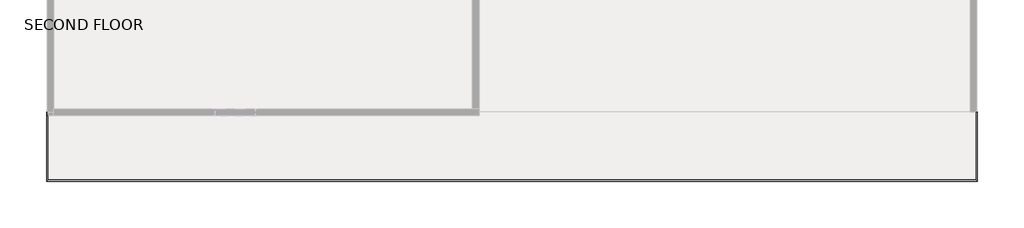
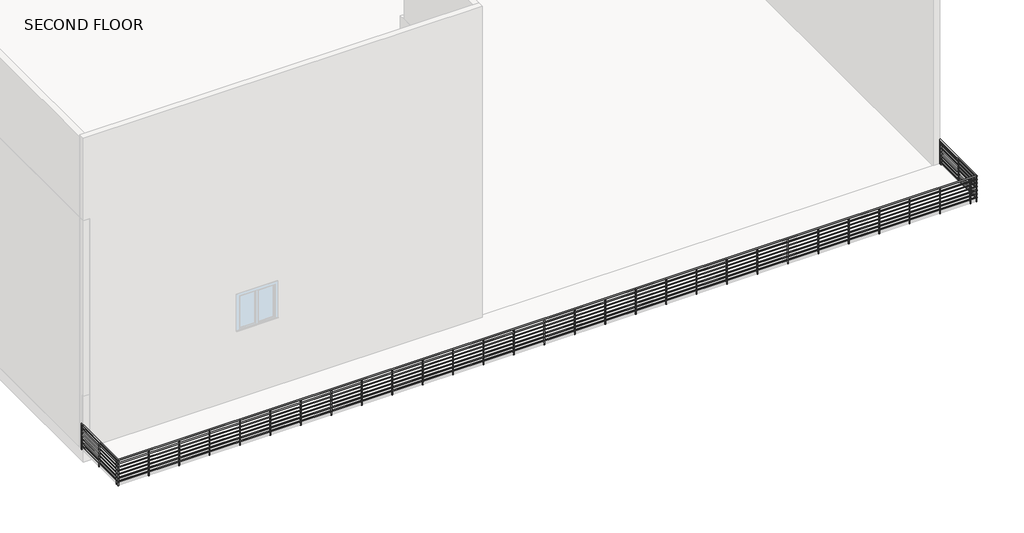
# One storey, part 2 of 2: 1 railing.
"""IFC4 building model written with IfcOpenShell, lengths in millimetres."""

from ifc_helpers import new_model, si_unit, point, frame, frame_2d, origin, place, context, project, spatial, circle_curve, ellipse_curve, trimmed, segment, composite_curve, outline, extrude, element, save
from ifc_brep_helpers import plane_surface, cylinder_surface, advanced_brep

model = new_model("IFC4")

# Units and contexts
model_context = context("Model", 3, world=origin())
ifc_project = project(units=[si_unit("LENGTHUNIT", "METRE", prefix="MILLI")], contexts=[model_context])

# Site, building, storey
site = spatial("IfcSite", under=ifc_project)
building = spatial("IfcBuilding", under=site)
storey = spatial("IfcBuildingStorey", under=building, Name="SECOND FLOOR", Elevation=6096.0)

# Railing
placement = place(None, origin())
element("IfcRailing", 1, ObjectType="900mm Pipe", at=placement, inside=storey, context=model_context, shape_type="SolidModel", body=[
    advanced_brep(
    [(-17910.01982, -7832.8965627, 6976.0), (-17870.01982, -7832.8965627, 6976.0), (-17910.01982, -9933.0763423, 6976.0), (-17870.01982, -9893.0763423, 6976.0), (10329.98018, -9933.0763423, 6976.0), (10289.98018, -9893.0763423, 6976.0), (10329.98018, -7832.8965627, 6976.0), (10289.98018, -7832.8965627, 6976.0)],
    [
        (0, 1, circle_curve(frame((-17890.01982, -7832.8965627, 6976.0), z_axis=(0.0, 1.0, 0.0), x_axis=(1.0, 0.0, 0.0)), 20.0)),
        (1, 0, circle_curve(frame((-17890.01982, -7832.8965627, 6976.0), z_axis=(0.0, 1.0, 0.0), x_axis=(1.0, 0.0, 0.0)), 20.0)),
        (0, 2),
        (2, 3, ellipse_curve(frame((-17890.01982, -9913.0763423, 6976.0), z_axis=(-0.7071067811865475, 0.7071067811865475, 0.0), x_axis=(0.7071067811865474, 0.7071067811865476, 0.0)), 28.2842712, 20.0)),
        (3, 1),
        (3, 2, ellipse_curve(frame((-17890.01982, -9913.0763423, 6976.0), z_axis=(-0.7071067811865475, 0.7071067811865475, 0.0), x_axis=(0.7071067811865474, 0.7071067811865476, 0.0)), 28.2842712, 20.0)),
        (2, 4),
        (4, 5, ellipse_curve(frame((10309.98018, -9913.0763423, 6976.0), z_axis=(-0.7071067811865475, -0.7071067811865475, 0.0), x_axis=(-0.7071067811865476, 0.7071067811865474, 0.0)), 28.2842712, 20.0)),
        (5, 3),
        (5, 4, ellipse_curve(frame((10309.98018, -9913.0763423, 6976.0), z_axis=(-0.7071067811865475, -0.7071067811865475, 0.0), x_axis=(-0.7071067811865476, 0.7071067811865474, 0.0)), 28.2842712, 20.0)),
        (6, 7, circle_curve(frame((10309.98018, -7832.8965627, 6976.0), z_axis=(0.0, 1.0, 0.0), x_axis=(-1.0, 0.0, 0.0)), 20.0)),
        (7, 6, circle_curve(frame((10309.98018, -7832.8965627, 6976.0), z_axis=(0.0, 1.0, 0.0), x_axis=(-1.0, 0.0, 0.0)), 20.0)),
        (4, 6),
        (7, 5),
    ],
    [
        plane_surface(frame((-17890.01982, -7832.8965627, 6996.0), z_axis=(0.0, 1.0, 0.0), x_axis=(0.0, 0.0, -1.0))),
        cylinder_surface(frame((-17890.01982, -7832.8965627, 6976.0), z_axis=(0.0, 1.0, 0.0), x_axis=(1.0, 0.0, 0.0)), 20.0),
        cylinder_surface(frame((-17890.01982, -9913.0763423, 6976.0), z_axis=(-1.0, 0.0, 0.0), x_axis=(0.0, 1.0, 0.0)), 20.0),
        plane_surface(frame((10309.98018, -7832.8965627, 6996.0), z_axis=(0.0, 1.0, 0.0), x_axis=(0.0, 0.0, 1.0))),
        cylinder_surface(frame((10309.98018, -9913.0763423, 6976.0), z_axis=(0.0, -1.0, 0.0), x_axis=(-1.0, 0.0, 0.0)), 20.0),
    ],
    [
        (0, [[1, 2]]),
        (1, [[-1, 3, 4, 5]]),
        (1, [[-2, -5, 6, -3]]),
        (2, [[-4, 7, 8, 9]]),
        (2, [[-6, -9, 10, -7]]),
        (3, [[11, 12]]),
        (4, [[-8, 13, -12, 14]]),
        (4, [[-10, -14, -11, -13]]),
    ],
),
    advanced_brep(
    [(-17875.01982, -7832.8965627, 6856.0), (-17905.01982, -7832.8965627, 6856.0), (-17875.01982, -9898.0763423, 6856.0), (-17905.01982, -9928.0763423, 6856.0), (10294.98018, -9898.0763423, 6856.0), (10324.98018, -9928.0763423, 6856.0), (10294.98018, -7832.8965627, 6856.0), (10324.98018, -7832.8965627, 6856.0)],
    [
        (0, 1, circle_curve(frame((-17890.01982, -7832.8965627, 6856.0), z_axis=(0.0, 1.0, 0.0), x_axis=(-1.0, 0.0, 0.0)), 15.0)),
        (1, 0, circle_curve(frame((-17890.01982, -7832.8965627, 6856.0), z_axis=(0.0, 1.0, 0.0), x_axis=(-1.0, 0.0, 0.0)), 15.0)),
        (0, 2),
        (2, 3, ellipse_curve(frame((-17890.01982, -9913.0763423, 6856.0), z_axis=(-0.7071067811865475, 0.7071067811865475, 0.0), x_axis=(0.7071067811865474, 0.7071067811865476, 0.0)), 21.2132034, 15.0)),
        (3, 1),
        (3, 2, ellipse_curve(frame((-17890.01982, -9913.0763423, 6856.0), z_axis=(-0.7071067811865475, 0.7071067811865475, 0.0), x_axis=(0.7071067811865474, 0.7071067811865476, 0.0)), 21.2132034, 15.0)),
        (2, 4),
        (4, 5, ellipse_curve(frame((10309.98018, -9913.0763423, 6856.0), z_axis=(-0.7071067811865475, -0.7071067811865475, 0.0), x_axis=(-0.7071067811865476, 0.7071067811865474, 0.0)), 21.2132034, 15.0)),
        (5, 3),
        (5, 4, ellipse_curve(frame((10309.98018, -9913.0763423, 6856.0), z_axis=(-0.7071067811865475, -0.7071067811865475, 0.0), x_axis=(-0.7071067811865476, 0.7071067811865474, 0.0)), 21.2132034, 15.0)),
        (6, 7, circle_curve(frame((10309.98018, -7832.8965627, 6856.0), z_axis=(0.0, 1.0, 0.0), x_axis=(1.0, 0.0, 0.0)), 15.0)),
        (7, 6, circle_curve(frame((10309.98018, -7832.8965627, 6856.0), z_axis=(0.0, 1.0, 0.0), x_axis=(1.0, 0.0, 0.0)), 15.0)),
        (4, 6),
        (7, 5),
    ],
    [
        plane_surface(frame((-17890.01982, -7832.8965627, 6871.0), z_axis=(0.0, 1.0, 0.0), x_axis=(0.0, 0.0, -1.0))),
        cylinder_surface(frame((-17890.01982, -7832.8965627, 6856.0), z_axis=(0.0, 1.0, 0.0), x_axis=(-1.0, 0.0, 0.0)), 15.0),
        cylinder_surface(frame((-17890.01982, -9913.0763423, 6856.0), z_axis=(-1.0, 0.0, 0.0), x_axis=(0.0, -1.0, 0.0)), 15.0),
        plane_surface(frame((10309.98018, -7832.8965627, 6871.0), z_axis=(0.0, 1.0, 0.0), x_axis=(0.0, 0.0, 1.0))),
        cylinder_surface(frame((10309.98018, -9913.0763423, 6856.0), z_axis=(0.0, -1.0, 0.0), x_axis=(1.0, 0.0, 0.0)), 15.0),
    ],
    [
        (0, [[1, 2]]),
        (1, [[-1, 3, 4, 5]]),
        (1, [[-2, -5, 6, -3]]),
        (2, [[-4, 7, 8, 9]]),
        (2, [[-6, -9, 10, -7]]),
        (3, [[11, 12]]),
        (4, [[-8, 13, -12, 14]]),
        (4, [[-10, -14, -11, -13]]),
    ],
),
    advanced_brep(
    [(-17875.01982, -7832.8965627, 6731.0), (-17905.01982, -7832.8965627, 6731.0), (-17875.01982, -9898.0763423, 6731.0), (-17905.01982, -9928.0763423, 6731.0), (10294.98018, -9898.0763423, 6731.0), (10324.98018, -9928.0763423, 6731.0), (10294.98018, -7832.8965627, 6731.0), (10324.98018, -7832.8965627, 6731.0)],
    [
        (0, 1, circle_curve(frame((-17890.01982, -7832.8965627, 6731.0), z_axis=(0.0, 1.0, 0.0), x_axis=(-1.0, 0.0, 0.0)), 15.0)),
        (1, 0, circle_curve(frame((-17890.01982, -7832.8965627, 6731.0), z_axis=(0.0, 1.0, 0.0), x_axis=(-1.0, 0.0, 0.0)), 15.0)),
        (0, 2),
        (2, 3, ellipse_curve(frame((-17890.01982, -9913.0763423, 6731.0), z_axis=(-0.7071067811865475, 0.7071067811865475, 0.0), x_axis=(0.7071067811865474, 0.7071067811865476, 0.0)), 21.2132034, 15.0)),
        (3, 1),
        (3, 2, ellipse_curve(frame((-17890.01982, -9913.0763423, 6731.0), z_axis=(-0.7071067811865475, 0.7071067811865475, 0.0), x_axis=(0.7071067811865474, 0.7071067811865476, 0.0)), 21.2132034, 15.0)),
        (2, 4),
        (4, 5, ellipse_curve(frame((10309.98018, -9913.0763423, 6731.0), z_axis=(-0.7071067811865475, -0.7071067811865475, 0.0), x_axis=(-0.7071067811865476, 0.7071067811865474, 0.0)), 21.2132034, 15.0)),
        (5, 3),
        (5, 4, ellipse_curve(frame((10309.98018, -9913.0763423, 6731.0), z_axis=(-0.7071067811865475, -0.7071067811865475, 0.0), x_axis=(-0.7071067811865476, 0.7071067811865474, 0.0)), 21.2132034, 15.0)),
        (6, 7, circle_curve(frame((10309.98018, -7832.8965627, 6731.0), z_axis=(0.0, 1.0, 0.0), x_axis=(1.0, 0.0, 0.0)), 15.0)),
        (7, 6, circle_curve(frame((10309.98018, -7832.8965627, 6731.0), z_axis=(0.0, 1.0, 0.0), x_axis=(1.0, 0.0, 0.0)), 15.0)),
        (4, 6),
        (7, 5),
    ],
    [
        plane_surface(frame((-17890.01982, -7832.8965627, 6746.0), z_axis=(0.0, 1.0, 0.0), x_axis=(0.0, 0.0, -1.0))),
        cylinder_surface(frame((-17890.01982, -7832.8965627, 6731.0), z_axis=(0.0, 1.0, 0.0), x_axis=(-1.0, 0.0, 0.0)), 15.0),
        cylinder_surface(frame((-17890.01982, -9913.0763423, 6731.0), z_axis=(-1.0, 0.0, 0.0), x_axis=(0.0, -1.0, 0.0)), 15.0),
        plane_surface(frame((10309.98018, -7832.8965627, 6746.0), z_axis=(0.0, 1.0, 0.0), x_axis=(0.0, 0.0, 1.0))),
        cylinder_surface(frame((10309.98018, -9913.0763423, 6731.0), z_axis=(0.0, -1.0, 0.0), x_axis=(1.0, 0.0, 0.0)), 15.0),
    ],
    [
        (0, [[1, 2]]),
        (1, [[-1, 3, 4, 5]]),
        (1, [[-2, -5, 6, -3]]),
        (2, [[-4, 7, 8, 9]]),
        (2, [[-6, -9, 10, -7]]),
        (3, [[11, 12]]),
        (4, [[-8, 13, -12, 14]]),
        (4, [[-10, -14, -11, -13]]),
    ],
),
    advanced_brep(
    [(-17875.01982, -7832.8965627, 6606.0), (-17905.01982, -7832.8965627, 6606.0), (-17875.01982, -9898.0763423, 6606.0), (-17905.01982, -9928.0763423, 6606.0), (10294.98018, -9898.0763423, 6606.0), (10324.98018, -9928.0763423, 6606.0), (10294.98018, -7832.8965627, 6606.0), (10324.98018, -7832.8965627, 6606.0)],
    [
        (0, 1, circle_curve(frame((-17890.01982, -7832.8965627, 6606.0), z_axis=(0.0, 1.0, 0.0), x_axis=(-1.0, 0.0, 0.0)), 15.0)),
        (1, 0, circle_curve(frame((-17890.01982, -7832.8965627, 6606.0), z_axis=(0.0, 1.0, 0.0), x_axis=(-1.0, 0.0, 0.0)), 15.0)),
        (0, 2),
        (2, 3, ellipse_curve(frame((-17890.01982, -9913.0763423, 6606.0), z_axis=(-0.7071067811865475, 0.7071067811865475, 0.0), x_axis=(0.7071067811865474, 0.7071067811865476, 0.0)), 21.2132034, 15.0)),
        (3, 1),
        (3, 2, ellipse_curve(frame((-17890.01982, -9913.0763423, 6606.0), z_axis=(-0.7071067811865475, 0.7071067811865475, 0.0), x_axis=(0.7071067811865474, 0.7071067811865476, 0.0)), 21.2132034, 15.0)),
        (2, 4),
        (4, 5, ellipse_curve(frame((10309.98018, -9913.0763423, 6606.0), z_axis=(-0.7071067811865475, -0.7071067811865475, 0.0), x_axis=(-0.7071067811865476, 0.7071067811865474, 0.0)), 21.2132034, 15.0)),
        (5, 3),
        (5, 4, ellipse_curve(frame((10309.98018, -9913.0763423, 6606.0), z_axis=(-0.7071067811865475, -0.7071067811865475, 0.0), x_axis=(-0.7071067811865476, 0.7071067811865474, 0.0)), 21.2132034, 15.0)),
        (6, 7, circle_curve(frame((10309.98018, -7832.8965627, 6606.0), z_axis=(0.0, 1.0, 0.0), x_axis=(1.0, 0.0, 0.0)), 15.0)),
        (7, 6, circle_curve(frame((10309.98018, -7832.8965627, 6606.0), z_axis=(0.0, 1.0, 0.0), x_axis=(1.0, 0.0, 0.0)), 15.0)),
        (4, 6),
        (7, 5),
    ],
    [
        plane_surface(frame((-17890.01982, -7832.8965627, 6621.0), z_axis=(0.0, 1.0, 0.0), x_axis=(0.0, 0.0, -1.0))),
        cylinder_surface(frame((-17890.01982, -7832.8965627, 6606.0), z_axis=(0.0, 1.0, 0.0), x_axis=(-1.0, 0.0, 0.0)), 15.0),
        cylinder_surface(frame((-17890.01982, -9913.0763423, 6606.0), z_axis=(-1.0, 0.0, 0.0), x_axis=(0.0, -1.0, 0.0)), 15.0),
        plane_surface(frame((10309.98018, -7832.8965627, 6621.0), z_axis=(0.0, 1.0, 0.0), x_axis=(0.0, 0.0, 1.0))),
        cylinder_surface(frame((10309.98018, -9913.0763423, 6606.0), z_axis=(0.0, -1.0, 0.0), x_axis=(1.0, 0.0, 0.0)), 15.0),
    ],
    [
        (0, [[1, 2]]),
        (1, [[-1, 3, 4, 5]]),
        (1, [[-2, -5, 6, -3]]),
        (2, [[-4, 7, 8, 9]]),
        (2, [[-6, -9, 10, -7]]),
        (3, [[11, 12]]),
        (4, [[-8, 13, -12, 14]]),
        (4, [[-10, -14, -11, -13]]),
    ],
),
    advanced_brep(
    [(-17875.01982, -7832.8965627, 6481.0), (-17905.01982, -7832.8965627, 6481.0), (-17875.01982, -9898.0763423, 6481.0), (-17905.01982, -9928.0763423, 6481.0), (10294.98018, -9898.0763423, 6481.0), (10324.98018, -9928.0763423, 6481.0), (10294.98018, -7832.8965627, 6481.0), (10324.98018, -7832.8965627, 6481.0)],
    [
        (0, 1, circle_curve(frame((-17890.01982, -7832.8965627, 6481.0), z_axis=(0.0, 1.0, 0.0), x_axis=(-1.0, 0.0, 0.0)), 15.0)),
        (1, 0, circle_curve(frame((-17890.01982, -7832.8965627, 6481.0), z_axis=(0.0, 1.0, 0.0), x_axis=(-1.0, 0.0, 0.0)), 15.0)),
        (0, 2),
        (2, 3, ellipse_curve(frame((-17890.01982, -9913.0763423, 6481.0), z_axis=(-0.7071067811865475, 0.7071067811865475, 0.0), x_axis=(0.7071067811865474, 0.7071067811865476, 0.0)), 21.2132034, 15.0)),
        (3, 1),
        (3, 2, ellipse_curve(frame((-17890.01982, -9913.0763423, 6481.0), z_axis=(-0.7071067811865475, 0.7071067811865475, 0.0), x_axis=(0.7071067811865474, 0.7071067811865476, 0.0)), 21.2132034, 15.0)),
        (2, 4),
        (4, 5, ellipse_curve(frame((10309.98018, -9913.0763423, 6481.0), z_axis=(-0.7071067811865475, -0.7071067811865475, 0.0), x_axis=(-0.7071067811865476, 0.7071067811865474, 0.0)), 21.2132034, 15.0)),
        (5, 3),
        (5, 4, ellipse_curve(frame((10309.98018, -9913.0763423, 6481.0), z_axis=(-0.7071067811865475, -0.7071067811865475, 0.0), x_axis=(-0.7071067811865476, 0.7071067811865474, 0.0)), 21.2132034, 15.0)),
        (6, 7, circle_curve(frame((10309.98018, -7832.8965627, 6481.0), z_axis=(0.0, 1.0, 0.0), x_axis=(1.0, 0.0, 0.0)), 15.0)),
        (7, 6, circle_curve(frame((10309.98018, -7832.8965627, 6481.0), z_axis=(0.0, 1.0, 0.0), x_axis=(1.0, 0.0, 0.0)), 15.0)),
        (4, 6),
        (7, 5),
    ],
    [
        plane_surface(frame((-17890.01982, -7832.8965627, 6496.0), z_axis=(0.0, 1.0, 0.0), x_axis=(0.0, 0.0, -1.0))),
        cylinder_surface(frame((-17890.01982, -7832.8965627, 6481.0), z_axis=(0.0, 1.0, 0.0), x_axis=(-1.0, 0.0, 0.0)), 15.0),
        cylinder_surface(frame((-17890.01982, -9913.0763423, 6481.0), z_axis=(-1.0, 0.0, 0.0), x_axis=(0.0, -1.0, 0.0)), 15.0),
        plane_surface(frame((10309.98018, -7832.8965627, 6496.0), z_axis=(0.0, 1.0, 0.0), x_axis=(0.0, 0.0, 1.0))),
        cylinder_surface(frame((10309.98018, -9913.0763423, 6481.0), z_axis=(0.0, -1.0, 0.0), x_axis=(1.0, 0.0, 0.0)), 15.0),
    ],
    [
        (0, [[1, 2]]),
        (1, [[-1, 3, 4, 5]]),
        (1, [[-2, -5, 6, -3]]),
        (2, [[-4, 7, 8, 9]]),
        (2, [[-6, -9, 10, -7]]),
        (3, [[11, 12]]),
        (4, [[-8, 13, -12, 14]]),
        (4, [[-10, -14, -11, -13]]),
    ],
),
    advanced_brep(
    [(-17875.01982, -7832.8965627, 6356.0), (-17905.01982, -7832.8965627, 6356.0), (-17875.01982, -9898.0763423, 6356.0), (-17905.01982, -9928.0763423, 6356.0), (10294.98018, -9898.0763423, 6356.0), (10324.98018, -9928.0763423, 6356.0), (10294.98018, -7832.8965627, 6356.0), (10324.98018, -7832.8965627, 6356.0)],
    [
        (0, 1, circle_curve(frame((-17890.01982, -7832.8965627, 6356.0), z_axis=(0.0, 1.0, 0.0), x_axis=(-1.0, 0.0, 0.0)), 15.0)),
        (1, 0, circle_curve(frame((-17890.01982, -7832.8965627, 6356.0), z_axis=(0.0, 1.0, 0.0), x_axis=(-1.0, 0.0, 0.0)), 15.0)),
        (0, 2),
        (2, 3, ellipse_curve(frame((-17890.01982, -9913.0763423, 6356.0), z_axis=(-0.7071067811865475, 0.7071067811865475, 0.0), x_axis=(0.7071067811865474, 0.7071067811865476, 0.0)), 21.2132034, 15.0)),
        (3, 1),
        (3, 2, ellipse_curve(frame((-17890.01982, -9913.0763423, 6356.0), z_axis=(-0.7071067811865475, 0.7071067811865475, 0.0), x_axis=(0.7071067811865474, 0.7071067811865476, 0.0)), 21.2132034, 15.0)),
        (2, 4),
        (4, 5, ellipse_curve(frame((10309.98018, -9913.0763423, 6356.0), z_axis=(-0.7071067811865475, -0.7071067811865475, 0.0), x_axis=(-0.7071067811865476, 0.7071067811865474, 0.0)), 21.2132034, 15.0)),
        (5, 3),
        (5, 4, ellipse_curve(frame((10309.98018, -9913.0763423, 6356.0), z_axis=(-0.7071067811865475, -0.7071067811865475, 0.0), x_axis=(-0.7071067811865476, 0.7071067811865474, 0.0)), 21.2132034, 15.0)),
        (6, 7, circle_curve(frame((10309.98018, -7832.8965627, 6356.0), z_axis=(0.0, 1.0, 0.0), x_axis=(1.0, 0.0, 0.0)), 15.0)),
        (7, 6, circle_curve(frame((10309.98018, -7832.8965627, 6356.0), z_axis=(0.0, 1.0, 0.0), x_axis=(1.0, 0.0, 0.0)), 15.0)),
        (4, 6),
        (7, 5),
    ],
    [
        plane_surface(frame((-17890.01982, -7832.8965627, 6371.0), z_axis=(0.0, 1.0, 0.0), x_axis=(0.0, 0.0, -1.0))),
        cylinder_surface(frame((-17890.01982, -7832.8965627, 6356.0), z_axis=(0.0, 1.0, 0.0), x_axis=(-1.0, 0.0, 0.0)), 15.0),
        cylinder_surface(frame((-17890.01982, -9913.0763423, 6356.0), z_axis=(-1.0, 0.0, 0.0), x_axis=(0.0, -1.0, 0.0)), 15.0),
        plane_surface(frame((10309.98018, -7832.8965627, 6371.0), z_axis=(0.0, 1.0, 0.0), x_axis=(0.0, 0.0, 1.0))),
        cylinder_surface(frame((10309.98018, -9913.0763423, 6356.0), z_axis=(0.0, -1.0, 0.0), x_axis=(1.0, 0.0, 0.0)), 15.0),
    ],
    [
        (0, [[1, 2]]),
        (1, [[-1, 3, 4, 5]]),
        (1, [[-2, -5, 6, -3]]),
        (2, [[-4, 7, 8, 9]]),
        (2, [[-6, -9, 10, -7]]),
        (3, [[11, 12]]),
        (4, [[-8, 13, -12, 14]]),
        (4, [[-10, -14, -11, -13]]),
    ],
),
    advanced_brep(
    [(-17875.01982, -7832.8965627, 6231.0), (-17905.01982, -7832.8965627, 6231.0), (-17875.01982, -9898.0763423, 6231.0), (-17905.01982, -9928.0763423, 6231.0), (10294.98018, -9898.0763423, 6231.0), (10324.98018, -9928.0763423, 6231.0), (10294.98018, -7832.8965627, 6231.0), (10324.98018, -7832.8965627, 6231.0)],
    [
        (0, 1, circle_curve(frame((-17890.01982, -7832.8965627, 6231.0), z_axis=(0.0, 1.0, 0.0), x_axis=(-1.0, 0.0, 0.0)), 15.0)),
        (1, 0, circle_curve(frame((-17890.01982, -7832.8965627, 6231.0), z_axis=(0.0, 1.0, 0.0), x_axis=(-1.0, 0.0, 0.0)), 15.0)),
        (0, 2),
        (2, 3, ellipse_curve(frame((-17890.01982, -9913.0763423, 6231.0), z_axis=(-0.7071067811865475, 0.7071067811865475, 0.0), x_axis=(0.7071067811865474, 0.7071067811865476, 0.0)), 21.2132034, 15.0)),
        (3, 1),
        (3, 2, ellipse_curve(frame((-17890.01982, -9913.0763423, 6231.0), z_axis=(-0.7071067811865475, 0.7071067811865475, 0.0), x_axis=(0.7071067811865474, 0.7071067811865476, 0.0)), 21.2132034, 15.0)),
        (2, 4),
        (4, 5, ellipse_curve(frame((10309.98018, -9913.0763423, 6231.0), z_axis=(-0.7071067811865475, -0.7071067811865475, 0.0), x_axis=(-0.7071067811865476, 0.7071067811865474, 0.0)), 21.2132034, 15.0)),
        (5, 3),
        (5, 4, ellipse_curve(frame((10309.98018, -9913.0763423, 6231.0), z_axis=(-0.7071067811865475, -0.7071067811865475, 0.0), x_axis=(-0.7071067811865476, 0.7071067811865474, 0.0)), 21.2132034, 15.0)),
        (6, 7, circle_curve(frame((10309.98018, -7832.8965627, 6231.0), z_axis=(0.0, 1.0, 0.0), x_axis=(1.0, 0.0, 0.0)), 15.0)),
        (7, 6, circle_curve(frame((10309.98018, -7832.8965627, 6231.0), z_axis=(0.0, 1.0, 0.0), x_axis=(1.0, 0.0, 0.0)), 15.0)),
        (4, 6),
        (7, 5),
    ],
    [
        plane_surface(frame((-17890.01982, -7832.8965627, 6246.0), z_axis=(0.0, 1.0, 0.0), x_axis=(0.0, 0.0, -1.0))),
        cylinder_surface(frame((-17890.01982, -7832.8965627, 6231.0), z_axis=(0.0, 1.0, 0.0), x_axis=(-1.0, 0.0, 0.0)), 15.0),
        cylinder_surface(frame((-17890.01982, -9913.0763423, 6231.0), z_axis=(-1.0, 0.0, 0.0), x_axis=(0.0, -1.0, 0.0)), 15.0),
        plane_surface(frame((10309.98018, -7832.8965627, 6246.0), z_axis=(0.0, 1.0, 0.0), x_axis=(0.0, 0.0, 1.0))),
        cylinder_surface(frame((10309.98018, -9913.0763423, 6231.0), z_axis=(0.0, -1.0, 0.0), x_axis=(1.0, 0.0, 0.0)), 15.0),
    ],
    [
        (0, [[1, 2]]),
        (1, [[-1, 3, 4, 5]]),
        (1, [[-2, -5, 6, -3]]),
        (2, [[-4, 7, 8, 9]]),
        (2, [[-6, -9, 10, -7]]),
        (3, [[11, 12]]),
        (4, [[-8, 13, -12, 14]]),
        (4, [[-10, -14, -11, -13]]),
    ],
),
    extrude(outline(composite_curve([segment(trimmed(circle_curve(frame_2d((10309.98018, -7913.0763423)), 12.5), [point((10297.48018, -7913.0763423))], [point((10322.48018, -7913.0763423))], False, "CARTESIAN"), True, "CONTINUOUS"), segment(trimmed(circle_curve(frame_2d((10309.98018, -7913.0763423)), 12.5), [point((10322.48018, -7913.0763423))], [point((10297.48018, -7913.0763423))], False, "CARTESIAN"), True, "CONTINUOUS")], self_intersect=False)), frame((0.0, 0.0, 6096.0), z_axis=(0.0, 0.0, 1.0), x_axis=(1.0, 0.0, 0.0)), (0.0, 0.0, 1.0), 860.0),
    extrude(outline(composite_curve([segment(trimmed(circle_curve(frame_2d((10309.98018, -8913.0763423)), 12.5), [point((10297.48018, -8913.0763423))], [point((10322.48018, -8913.0763423))], False, "CARTESIAN"), True, "CONTINUOUS"), segment(trimmed(circle_curve(frame_2d((10309.98018, -8913.0763423)), 12.5), [point((10322.48018, -8913.0763423))], [point((10297.48018, -8913.0763423))], False, "CARTESIAN"), True, "CONTINUOUS")], self_intersect=False)), frame((0.0, 0.0, 6096.0), z_axis=(0.0, 0.0, 1.0), x_axis=(1.0, 0.0, 0.0)), (0.0, 0.0, 1.0), 860.0),
    extrude(outline(composite_curve([segment(trimmed(circle_curve(frame_2d((10109.98018, -9913.0763423)), 12.5), [point((10109.98018, -9900.5763423))], [point((10109.98018, -9925.5763423))], False, "CARTESIAN"), True, "CONTINUOUS"), segment(trimmed(circle_curve(frame_2d((10109.98018, -9913.0763423)), 12.5), [point((10109.98018, -9925.5763423))], [point((10109.98018, -9900.5763423))], False, "CARTESIAN"), True, "CONTINUOUS")], self_intersect=False)), frame((0.0, 0.0, 6096.0), z_axis=(0.0, 0.0, 1.0), x_axis=(1.0, 0.0, 0.0)), (0.0, 0.0, 1.0), 860.0),
    extrude(outline(composite_curve([segment(trimmed(circle_curve(frame_2d((9109.98018, -9913.0763423)), 12.5), [point((9109.98018, -9900.5763423))], [point((9109.98018, -9925.5763423))], False, "CARTESIAN"), True, "CONTINUOUS"), segment(trimmed(circle_curve(frame_2d((9109.98018, -9913.0763423)), 12.5), [point((9109.98018, -9925.5763423))], [point((9109.98018, -9900.5763423))], False, "CARTESIAN"), True, "CONTINUOUS")], self_intersect=False)), frame((0.0, 0.0, 6096.0), z_axis=(0.0, 0.0, 1.0), x_axis=(1.0, 0.0, 0.0)), (0.0, 0.0, 1.0), 860.0),
    extrude(outline(composite_curve([segment(trimmed(circle_curve(frame_2d((8109.98018, -9913.0763423)), 12.5), [point((8109.98018, -9900.5763423))], [point((8109.98018, -9925.5763423))], False, "CARTESIAN"), True, "CONTINUOUS"), segment(trimmed(circle_curve(frame_2d((8109.98018, -9913.0763423)), 12.5), [point((8109.98018, -9925.5763423))], [point((8109.98018, -9900.5763423))], False, "CARTESIAN"), True, "CONTINUOUS")], self_intersect=False)), frame((0.0, 0.0, 6096.0), z_axis=(0.0, 0.0, 1.0), x_axis=(1.0, 0.0, 0.0)), (0.0, 0.0, 1.0), 860.0),
    extrude(outline(composite_curve([segment(trimmed(circle_curve(frame_2d((7109.98018, -9913.0763423)), 12.5), [point((7109.98018, -9900.5763423))], [point((7109.98018, -9925.5763423))], False, "CARTESIAN"), True, "CONTINUOUS"), segment(trimmed(circle_curve(frame_2d((7109.98018, -9913.0763423)), 12.5), [point((7109.98018, -9925.5763423))], [point((7109.98018, -9900.5763423))], False, "CARTESIAN"), True, "CONTINUOUS")], self_intersect=False)), frame((0.0, 0.0, 6096.0), z_axis=(0.0, 0.0, 1.0), x_axis=(1.0, 0.0, 0.0)), (0.0, 0.0, 1.0), 860.0),
    extrude(outline(composite_curve([segment(trimmed(circle_curve(frame_2d((6109.98018, -9913.0763423)), 12.5), [point((6109.98018, -9900.5763423))], [point((6109.98018, -9925.5763423))], False, "CARTESIAN"), True, "CONTINUOUS"), segment(trimmed(circle_curve(frame_2d((6109.98018, -9913.0763423)), 12.5), [point((6109.98018, -9925.5763423))], [point((6109.98018, -9900.5763423))], False, "CARTESIAN"), True, "CONTINUOUS")], self_intersect=False)), frame((0.0, 0.0, 6096.0), z_axis=(0.0, 0.0, 1.0), x_axis=(1.0, 0.0, 0.0)), (0.0, 0.0, 1.0), 860.0),
    extrude(outline(composite_curve([segment(trimmed(circle_curve(frame_2d((5109.98018, -9913.0763423)), 12.5), [point((5109.98018, -9900.5763423))], [point((5109.98018, -9925.5763423))], False, "CARTESIAN"), True, "CONTINUOUS"), segment(trimmed(circle_curve(frame_2d((5109.98018, -9913.0763423)), 12.5), [point((5109.98018, -9925.5763423))], [point((5109.98018, -9900.5763423))], False, "CARTESIAN"), True, "CONTINUOUS")], self_intersect=False)), frame((0.0, 0.0, 6096.0), z_axis=(0.0, 0.0, 1.0), x_axis=(1.0, 0.0, 0.0)), (0.0, 0.0, 1.0), 860.0),
    extrude(outline(composite_curve([segment(trimmed(circle_curve(frame_2d((4109.98018, -9913.0763423)), 12.5), [point((4109.98018, -9900.5763423))], [point((4109.98018, -9925.5763423))], False, "CARTESIAN"), True, "CONTINUOUS"), segment(trimmed(circle_curve(frame_2d((4109.98018, -9913.0763423)), 12.5), [point((4109.98018, -9925.5763423))], [point((4109.98018, -9900.5763423))], False, "CARTESIAN"), True, "CONTINUOUS")], self_intersect=False)), frame((0.0, 0.0, 6096.0), z_axis=(0.0, 0.0, 1.0), x_axis=(1.0, 0.0, 0.0)), (0.0, 0.0, 1.0), 860.0),
    extrude(outline(composite_curve([segment(trimmed(circle_curve(frame_2d((3109.98018, -9913.0763423)), 12.5), [point((3109.98018, -9900.5763423))], [point((3109.98018, -9925.5763423))], False, "CARTESIAN"), True, "CONTINUOUS"), segment(trimmed(circle_curve(frame_2d((3109.98018, -9913.0763423)), 12.5), [point((3109.98018, -9925.5763423))], [point((3109.98018, -9900.5763423))], False, "CARTESIAN"), True, "CONTINUOUS")], self_intersect=False)), frame((0.0, 0.0, 6096.0), z_axis=(0.0, 0.0, 1.0), x_axis=(1.0, 0.0, 0.0)), (0.0, 0.0, 1.0), 860.0),
    extrude(outline(composite_curve([segment(trimmed(circle_curve(frame_2d((2109.98018, -9913.0763423)), 12.5), [point((2109.98018, -9900.5763423))], [point((2109.98018, -9925.5763423))], False, "CARTESIAN"), True, "CONTINUOUS"), segment(trimmed(circle_curve(frame_2d((2109.98018, -9913.0763423)), 12.5), [point((2109.98018, -9925.5763423))], [point((2109.98018, -9900.5763423))], False, "CARTESIAN"), True, "CONTINUOUS")], self_intersect=False)), frame((0.0, 0.0, 6096.0), z_axis=(0.0, 0.0, 1.0), x_axis=(1.0, 0.0, 0.0)), (0.0, 0.0, 1.0), 860.0),
    extrude(outline(composite_curve([segment(trimmed(circle_curve(frame_2d((1109.98018, -9913.0763423)), 12.5), [point((1109.98018, -9900.5763423))], [point((1109.98018, -9925.5763423))], False, "CARTESIAN"), True, "CONTINUOUS"), segment(trimmed(circle_curve(frame_2d((1109.98018, -9913.0763423)), 12.5), [point((1109.98018, -9925.5763423))], [point((1109.98018, -9900.5763423))], False, "CARTESIAN"), True, "CONTINUOUS")], self_intersect=False)), frame((0.0, 0.0, 6096.0), z_axis=(0.0, 0.0, 1.0), x_axis=(1.0, 0.0, 0.0)), (0.0, 0.0, 1.0), 860.0),
    extrude(outline(composite_curve([segment(trimmed(circle_curve(frame_2d((109.98018, -9913.0763423)), 12.5), [point((109.98018, -9900.5763423))], [point((109.98018, -9925.5763423))], False, "CARTESIAN"), True, "CONTINUOUS"), segment(trimmed(circle_curve(frame_2d((109.98018, -9913.0763423)), 12.5), [point((109.98018, -9925.5763423))], [point((109.98018, -9900.5763423))], False, "CARTESIAN"), True, "CONTINUOUS")], self_intersect=False)), frame((0.0, 0.0, 6096.0), z_axis=(0.0, 0.0, 1.0), x_axis=(1.0, 0.0, 0.0)), (0.0, 0.0, 1.0), 860.0),
    extrude(outline(composite_curve([segment(trimmed(circle_curve(frame_2d((-890.01982, -9913.0763423)), 12.5), [point((-890.01982, -9900.5763423))], [point((-890.01982, -9925.5763423))], False, "CARTESIAN"), True, "CONTINUOUS"), segment(trimmed(circle_curve(frame_2d((-890.01982, -9913.0763423)), 12.5), [point((-890.01982, -9925.5763423))], [point((-890.01982, -9900.5763423))], False, "CARTESIAN"), True, "CONTINUOUS")], self_intersect=False)), frame((0.0, 0.0, 6096.0), z_axis=(0.0, 0.0, 1.0), x_axis=(1.0, 0.0, 0.0)), (0.0, 0.0, 1.0), 860.0),
    extrude(outline(composite_curve([segment(trimmed(circle_curve(frame_2d((-1890.01982, -9913.0763423)), 12.5), [point((-1890.01982, -9900.5763423))], [point((-1890.01982, -9925.5763423))], False, "CARTESIAN"), True, "CONTINUOUS"), segment(trimmed(circle_curve(frame_2d((-1890.01982, -9913.0763423)), 12.5), [point((-1890.01982, -9925.5763423))], [point((-1890.01982, -9900.5763423))], False, "CARTESIAN"), True, "CONTINUOUS")], self_intersect=False)), frame((0.0, 0.0, 6096.0), z_axis=(0.0, 0.0, 1.0), x_axis=(1.0, 0.0, 0.0)), (0.0, 0.0, 1.0), 860.0),
    extrude(outline(composite_curve([segment(trimmed(circle_curve(frame_2d((-2890.01982, -9913.0763423)), 12.5), [point((-2890.01982, -9900.5763423))], [point((-2890.01982, -9925.5763423))], False, "CARTESIAN"), True, "CONTINUOUS"), segment(trimmed(circle_curve(frame_2d((-2890.01982, -9913.0763423)), 12.5), [point((-2890.01982, -9925.5763423))], [point((-2890.01982, -9900.5763423))], False, "CARTESIAN"), True, "CONTINUOUS")], self_intersect=False)), frame((0.0, 0.0, 6096.0), z_axis=(0.0, 0.0, 1.0), x_axis=(1.0, 0.0, 0.0)), (0.0, 0.0, 1.0), 860.0),
    extrude(outline(composite_curve([segment(trimmed(circle_curve(frame_2d((-3890.01982, -9913.0763423)), 12.5), [point((-3890.01982, -9900.5763423))], [point((-3890.01982, -9925.5763423))], False, "CARTESIAN"), True, "CONTINUOUS"), segment(trimmed(circle_curve(frame_2d((-3890.01982, -9913.0763423)), 12.5), [point((-3890.01982, -9925.5763423))], [point((-3890.01982, -9900.5763423))], False, "CARTESIAN"), True, "CONTINUOUS")], self_intersect=False)), frame((0.0, 0.0, 6096.0), z_axis=(0.0, 0.0, 1.0), x_axis=(1.0, 0.0, 0.0)), (0.0, 0.0, 1.0), 860.0),
    extrude(outline(composite_curve([segment(trimmed(circle_curve(frame_2d((-4890.01982, -9913.0763423)), 12.5), [point((-4890.01982, -9900.5763423))], [point((-4890.01982, -9925.5763423))], False, "CARTESIAN"), True, "CONTINUOUS"), segment(trimmed(circle_curve(frame_2d((-4890.01982, -9913.0763423)), 12.5), [point((-4890.01982, -9925.5763423))], [point((-4890.01982, -9900.5763423))], False, "CARTESIAN"), True, "CONTINUOUS")], self_intersect=False)), frame((0.0, 0.0, 6096.0), z_axis=(0.0, 0.0, 1.0), x_axis=(1.0, 0.0, 0.0)), (0.0, 0.0, 1.0), 860.0),
    extrude(outline(composite_curve([segment(trimmed(circle_curve(frame_2d((-5890.01982, -9913.0763423)), 12.5), [point((-5890.01982, -9900.5763423))], [point((-5890.01982, -9925.5763423))], False, "CARTESIAN"), True, "CONTINUOUS"), segment(trimmed(circle_curve(frame_2d((-5890.01982, -9913.0763423)), 12.5), [point((-5890.01982, -9925.5763423))], [point((-5890.01982, -9900.5763423))], False, "CARTESIAN"), True, "CONTINUOUS")], self_intersect=False)), frame((0.0, 0.0, 6096.0), z_axis=(0.0, 0.0, 1.0), x_axis=(1.0, 0.0, 0.0)), (0.0, 0.0, 1.0), 860.0),
    extrude(outline(composite_curve([segment(trimmed(circle_curve(frame_2d((-6890.01982, -9913.0763423)), 12.5), [point((-6890.01982, -9900.5763423))], [point((-6890.01982, -9925.5763423))], False, "CARTESIAN"), True, "CONTINUOUS"), segment(trimmed(circle_curve(frame_2d((-6890.01982, -9913.0763423)), 12.5), [point((-6890.01982, -9925.5763423))], [point((-6890.01982, -9900.5763423))], False, "CARTESIAN"), True, "CONTINUOUS")], self_intersect=False)), frame((0.0, 0.0, 6096.0), z_axis=(0.0, 0.0, 1.0), x_axis=(1.0, 0.0, 0.0)), (0.0, 0.0, 1.0), 860.0),
    extrude(outline(composite_curve([segment(trimmed(circle_curve(frame_2d((-7890.01982, -9913.0763423)), 12.5), [point((-7890.01982, -9900.5763423))], [point((-7890.01982, -9925.5763423))], False, "CARTESIAN"), True, "CONTINUOUS"), segment(trimmed(circle_curve(frame_2d((-7890.01982, -9913.0763423)), 12.5), [point((-7890.01982, -9925.5763423))], [point((-7890.01982, -9900.5763423))], False, "CARTESIAN"), True, "CONTINUOUS")], self_intersect=False)), frame((0.0, 0.0, 6096.0), z_axis=(0.0, 0.0, 1.0), x_axis=(1.0, 0.0, 0.0)), (0.0, 0.0, 1.0), 860.0),
    extrude(outline(composite_curve([segment(trimmed(circle_curve(frame_2d((-8890.01982, -9913.0763423)), 12.5), [point((-8890.01982, -9900.5763423))], [point((-8890.01982, -9925.5763423))], False, "CARTESIAN"), True, "CONTINUOUS"), segment(trimmed(circle_curve(frame_2d((-8890.01982, -9913.0763423)), 12.5), [point((-8890.01982, -9925.5763423))], [point((-8890.01982, -9900.5763423))], False, "CARTESIAN"), True, "CONTINUOUS")], self_intersect=False)), frame((0.0, 0.0, 6096.0), z_axis=(0.0, 0.0, 1.0), x_axis=(1.0, 0.0, 0.0)), (0.0, 0.0, 1.0), 860.0),
    extrude(outline(composite_curve([segment(trimmed(circle_curve(frame_2d((-9890.01982, -9913.0763423)), 12.5), [point((-9890.01982, -9900.5763423))], [point((-9890.01982, -9925.5763423))], False, "CARTESIAN"), True, "CONTINUOUS"), segment(trimmed(circle_curve(frame_2d((-9890.01982, -9913.0763423)), 12.5), [point((-9890.01982, -9925.5763423))], [point((-9890.01982, -9900.5763423))], False, "CARTESIAN"), True, "CONTINUOUS")], self_intersect=False)), frame((0.0, 0.0, 6096.0), z_axis=(0.0, 0.0, 1.0), x_axis=(1.0, 0.0, 0.0)), (0.0, 0.0, 1.0), 860.0),
    extrude(outline(composite_curve([segment(trimmed(circle_curve(frame_2d((-10890.01982, -9913.0763423)), 12.5), [point((-10890.01982, -9900.5763423))], [point((-10890.01982, -9925.5763423))], False, "CARTESIAN"), True, "CONTINUOUS"), segment(trimmed(circle_curve(frame_2d((-10890.01982, -9913.0763423)), 12.5), [point((-10890.01982, -9925.5763423))], [point((-10890.01982, -9900.5763423))], False, "CARTESIAN"), True, "CONTINUOUS")], self_intersect=False)), frame((0.0, 0.0, 6096.0), z_axis=(0.0, 0.0, 1.0), x_axis=(1.0, 0.0, 0.0)), (0.0, 0.0, 1.0), 860.0),
    extrude(outline(composite_curve([segment(trimmed(circle_curve(frame_2d((-11890.01982, -9913.0763423)), 12.5), [point((-11890.01982, -9900.5763423))], [point((-11890.01982, -9925.5763423))], False, "CARTESIAN"), True, "CONTINUOUS"), segment(trimmed(circle_curve(frame_2d((-11890.01982, -9913.0763423)), 12.5), [point((-11890.01982, -9925.5763423))], [point((-11890.01982, -9900.5763423))], False, "CARTESIAN"), True, "CONTINUOUS")], self_intersect=False)), frame((0.0, 0.0, 6096.0), z_axis=(0.0, 0.0, 1.0), x_axis=(1.0, 0.0, 0.0)), (0.0, 0.0, 1.0), 860.0),
    extrude(outline(composite_curve([segment(trimmed(circle_curve(frame_2d((-12890.01982, -9913.0763423)), 12.5), [point((-12890.01982, -9900.5763423))], [point((-12890.01982, -9925.5763423))], False, "CARTESIAN"), True, "CONTINUOUS"), segment(trimmed(circle_curve(frame_2d((-12890.01982, -9913.0763423)), 12.5), [point((-12890.01982, -9925.5763423))], [point((-12890.01982, -9900.5763423))], False, "CARTESIAN"), True, "CONTINUOUS")], self_intersect=False)), frame((0.0, 0.0, 6096.0), z_axis=(0.0, 0.0, 1.0), x_axis=(1.0, 0.0, 0.0)), (0.0, 0.0, 1.0), 860.0),
    extrude(outline(composite_curve([segment(trimmed(circle_curve(frame_2d((-13890.01982, -9913.0763423)), 12.5), [point((-13890.01982, -9900.5763423))], [point((-13890.01982, -9925.5763423))], False, "CARTESIAN"), True, "CONTINUOUS"), segment(trimmed(circle_curve(frame_2d((-13890.01982, -9913.0763423)), 12.5), [point((-13890.01982, -9925.5763423))], [point((-13890.01982, -9900.5763423))], False, "CARTESIAN"), True, "CONTINUOUS")], self_intersect=False)), frame((0.0, 0.0, 6096.0), z_axis=(0.0, 0.0, 1.0), x_axis=(1.0, 0.0, 0.0)), (0.0, 0.0, 1.0), 860.0),
    extrude(outline(composite_curve([segment(trimmed(circle_curve(frame_2d((-14890.01982, -9913.0763423)), 12.5), [point((-14890.01982, -9900.5763423))], [point((-14890.01982, -9925.5763423))], False, "CARTESIAN"), True, "CONTINUOUS"), segment(trimmed(circle_curve(frame_2d((-14890.01982, -9913.0763423)), 12.5), [point((-14890.01982, -9925.5763423))], [point((-14890.01982, -9900.5763423))], False, "CARTESIAN"), True, "CONTINUOUS")], self_intersect=False)), frame((0.0, 0.0, 6096.0), z_axis=(0.0, 0.0, 1.0), x_axis=(1.0, 0.0, 0.0)), (0.0, 0.0, 1.0), 860.0),
    extrude(outline(composite_curve([segment(trimmed(circle_curve(frame_2d((-15890.01982, -9913.0763423)), 12.5), [point((-15890.01982, -9900.5763423))], [point((-15890.01982, -9925.5763423))], False, "CARTESIAN"), True, "CONTINUOUS"), segment(trimmed(circle_curve(frame_2d((-15890.01982, -9913.0763423)), 12.5), [point((-15890.01982, -9925.5763423))], [point((-15890.01982, -9900.5763423))], False, "CARTESIAN"), True, "CONTINUOUS")], self_intersect=False)), frame((0.0, 0.0, 6096.0), z_axis=(0.0, 0.0, 1.0), x_axis=(1.0, 0.0, 0.0)), (0.0, 0.0, 1.0), 860.0),
    extrude(outline(composite_curve([segment(trimmed(circle_curve(frame_2d((-16890.01982, -9913.0763423)), 12.5), [point((-16890.01982, -9900.5763423))], [point((-16890.01982, -9925.5763423))], False, "CARTESIAN"), True, "CONTINUOUS"), segment(trimmed(circle_curve(frame_2d((-16890.01982, -9913.0763423)), 12.5), [point((-16890.01982, -9925.5763423))], [point((-16890.01982, -9900.5763423))], False, "CARTESIAN"), True, "CONTINUOUS")], self_intersect=False)), frame((0.0, 0.0, 6096.0), z_axis=(0.0, 0.0, 1.0), x_axis=(1.0, 0.0, 0.0)), (0.0, 0.0, 1.0), 860.0),
    extrude(outline(composite_curve([segment(trimmed(circle_curve(frame_2d((-17890.01982, -9832.8965627)), 12.5), [point((-17877.51982, -9832.8965627))], [point((-17902.51982, -9832.8965627))], False, "CARTESIAN"), True, "CONTINUOUS"), segment(trimmed(circle_curve(frame_2d((-17890.01982, -9832.8965627)), 12.5), [point((-17902.51982, -9832.8965627))], [point((-17877.51982, -9832.8965627))], False, "CARTESIAN"), True, "CONTINUOUS")], self_intersect=False)), frame((0.0, 0.0, 6096.0), z_axis=(0.0, 0.0, 1.0), x_axis=(1.0, 0.0, 0.0)), (0.0, 0.0, 1.0), 860.0),
    extrude(outline(composite_curve([segment(trimmed(circle_curve(frame_2d((-17890.01982, -8832.8965627)), 12.5), [point((-17877.51982, -8832.8965627))], [point((-17902.51982, -8832.8965627))], False, "CARTESIAN"), True, "CONTINUOUS"), segment(trimmed(circle_curve(frame_2d((-17890.01982, -8832.8965627)), 12.5), [point((-17902.51982, -8832.8965627))], [point((-17877.51982, -8832.8965627))], False, "CARTESIAN"), True, "CONTINUOUS")], self_intersect=False)), frame((0.0, 0.0, 6096.0), z_axis=(0.0, 0.0, 1.0), x_axis=(1.0, 0.0, 0.0)), (0.0, 0.0, 1.0), 860.0),
    extrude(outline(composite_curve([segment(trimmed(circle_curve(frame_2d((10309.98018, -9913.0763423)), 12.5), [point((10309.98018, -9900.5763423))], [point((10309.98018, -9925.5763423))], False, "CARTESIAN"), True, "CONTINUOUS"), segment(trimmed(circle_curve(frame_2d((10309.98018, -9913.0763423)), 12.5), [point((10309.98018, -9925.5763423))], [point((10309.98018, -9900.5763423))], False, "CARTESIAN"), True, "CONTINUOUS")], self_intersect=False)), frame((0.0, 0.0, 6096.0), z_axis=(0.0, 0.0, 1.0), x_axis=(1.0, 0.0, 0.0)), (0.0, 0.0, 1.0), 860.0),
    extrude(outline(composite_curve([segment(trimmed(circle_curve(frame_2d((-17890.01982, -9913.0763423)), 12.5), [point((-17877.51982, -9913.0763423))], [point((-17902.51982, -9913.0763423))], False, "CARTESIAN"), True, "CONTINUOUS"), segment(trimmed(circle_curve(frame_2d((-17890.01982, -9913.0763423)), 12.5), [point((-17902.51982, -9913.0763423))], [point((-17877.51982, -9913.0763423))], False, "CARTESIAN"), True, "CONTINUOUS")], self_intersect=False)), frame((0.0, 0.0, 6096.0), z_axis=(0.0, 0.0, 1.0), x_axis=(1.0, 0.0, 0.0)), (0.0, 0.0, 1.0), 860.0),
    extrude(outline(composite_curve([segment(trimmed(circle_curve(frame_2d((10309.98018, -7845.3965627)), 12.5), [point((10297.48018, -7845.3965627))], [point((10322.48018, -7845.3965627))], False, "CARTESIAN"), True, "CONTINUOUS"), segment(trimmed(circle_curve(frame_2d((10309.98018, -7845.3965627)), 12.5), [point((10322.48018, -7845.3965627))], [point((10297.48018, -7845.3965627))], False, "CARTESIAN"), True, "CONTINUOUS")], self_intersect=False)), frame((0.0, 0.0, 6096.0), z_axis=(0.0, 0.0, 1.0), x_axis=(1.0, 0.0, 0.0)), (0.0, 0.0, 1.0), 860.0),
    extrude(outline(composite_curve([segment(trimmed(circle_curve(frame_2d((-17890.01982, -7845.3965627)), 12.5), [point((-17877.51982, -7845.3965627))], [point((-17902.51982, -7845.3965627))], False, "CARTESIAN"), True, "CONTINUOUS"), segment(trimmed(circle_curve(frame_2d((-17890.01982, -7845.3965627)), 12.5), [point((-17902.51982, -7845.3965627))], [point((-17877.51982, -7845.3965627))], False, "CARTESIAN"), True, "CONTINUOUS")], self_intersect=False)), frame((0.0, 0.0, 6096.0), z_axis=(0.0, 0.0, 1.0), x_axis=(1.0, 0.0, 0.0)), (0.0, 0.0, 1.0), 860.0),
])

save(model, "model.ifc")

# Revit data of these elements
# Type "900mm Pipe"
#   built-in parameter 1008612 = 0.019685 (stored number, unit not read)
#   built-in parameter 1008611 = 0.0984252 (stored number, unit not read)
#   built-in parameter 1008609 = 6.56168 (stored number, unit not read)
#   built-in parameter 1008604 = 0.19685 (stored number, unit not read)
#   built-in parameter 1008603 = 0.164042 (stored number, unit not read)
#   Railing Height = 2' - 11.43307"
#   built-in parameter 1008630 = 2
#   built-in parameter 1008610 = 2
#   built-in parameter 1008605 = 1
#   built-in parameter 1008618 = M_Baluster - Round : 25mm
# Element 1 (IfcRailing, "900mm Pipe")
#   Phase Created = New Construction
